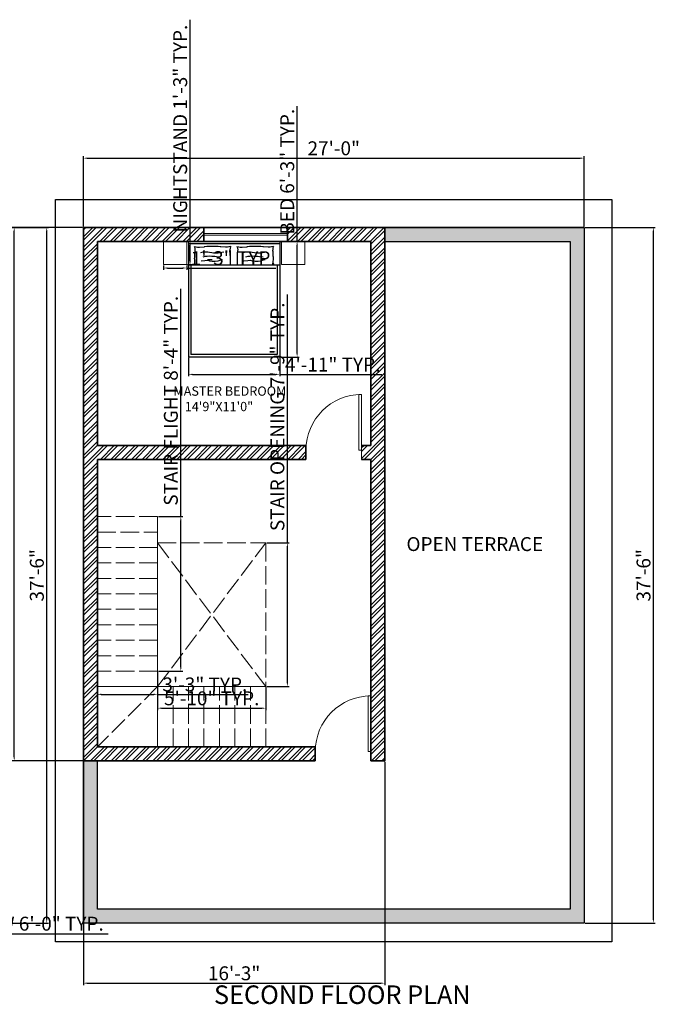
# Model space of a CAD drawing. Units: inches. Extents: x 638 to 1853, y 4393 to 5041.
# Tile 6 of 6: x 1441 to 1853, y 4404 to 5041. Entities that reach past the tile are written whole.
import ezdxf

# ---------------------------------------------------------------- set-up
doc = ezdxf.new("R2010")
doc.units = ezdxf.units.IN
doc.linetypes.add('ACAD_ISO02W100', pattern=[15, 12, -3])
for name, color, linetype, lineweight in [('A-ANNO-DIMS', 2, 'Continuous', 18), ('A-ANNO-TEXT', 7, 'Continuous', 25), ('A-AREA-IDEN', 7, 'Continuous', 18), ('A-DOOR', 4, 'Continuous', 18), ('A-FLOR-STRS', 7, 'Continuous', 18), ('A-FLOR-STRS-HIDN', 7, 'ACAD_ISO02W100', 18), ('A-FURN', 26, 'Continuous', 13), ('A-GLAZ', 5, 'Continuous', 18), ('A-WALL', 7, 'Continuous', 35), ('A-WALL-PATT', 251, 'Continuous', 13), ('A-WALL-PRPT', 7, 'Continuous', 25), ('A-WALL-PRPT-PATT', 141, 'Continuous', 13), ('C-PROP', 7, 'Continuous', 25)]:
    doc.layers.add(name, color=color, linetype=linetype, lineweight=lineweight)
doc.layers.add('supurgelik', color=31, linetype='Continuous')
doc.layers.add('TASLAR', color=32, linetype='Continuous')
doc.styles.get("Standard").update_dxf_attribs({"font": 'arial.ttf'})
doc.dimstyles.new('ISO-25', dxfattribs={"dimtxt": 9, "dimasz": 2.5, "dimexe": 1.25, "dimexo": 0.625, "dimtad": 1, "dimdec": 1, "dimlunit": 3, "dimtxsty": 'Standard', "dimcen": 2.5, "dimadec": 0, "dimazin": 0, "dimtfac": 1, "dimtdec": 1, "dimtmove": 0, "dimatfit": 3, "dimfxl": 1, "dimarcsym": 0})

# ---------------------------------------------------------------- blocks, each defined once
blk = doc.blocks.new('*U2')
for p, q in [((0, 0), (0, -6)), ((-36, 0), (-36, -6))]:
    blk.add_line(p, q)
blk.add_lwpolyline([(0, 0), (0, 36), (-1.75, 36), (-1.75, 0)], close=True)
blk.add_arc((0, 0), 36, 90, 180)
blk = doc.blocks.new('hgjgh')
at = {"layer": 'supurgelik'}
for p, q in [((85993.8, -4751.9), (85843.8, -4751.9)), ((85853.3, -4756.1), (85856.3, -4757)), ((85853.3, -4756.1), (85854.2, -4758.5)), ((85854.2, -4758.5), (85854.5, -4762.2)), ((85856.3, -4757), (85858.5, -4757.5)), ((85858.5, -4757.5), (85862.1, -4757.4)), ((85862.1, -4757.4), (85869.6, -4756.7)), ((85864.2, -4765.9), (85867.9, -4765)), ((85867.9, -4765), (85871.9, -4764.9)), ((85871.9, -4764.9), (85875.4, -4765.1)), ((85875.4, -4765.1), (85878.5, -4765.7)), ((85878.5, -4765.7), (85882, -4766.2)), ((85882, -4766.2), (85884.8, -4766.6)), ((85884.8, -4766.6), (85888.7, -4766.9)), ((85888.7, -4766.9), (85892.6, -4766.9)), ((85892.6, -4766.9), (85895.1, -4766.4)), ((85895.1, -4766.4), (85901.8, -4764.9)), ((85904.4, -4757.4), (85897, -4756.7)), ((85908, -4757.5), (85904.4, -4757.4)), ((85910.2, -4757), (85908, -4757.5)), ((85913.3, -4756.1), (85910.2, -4757)), ((85912.3, -4758.5), (85912, -4762.2)), ((85913.3, -4756.1), (85912.3, -4758.5)), ((85923.5, -4756.1), (85926.5, -4757)), ((85923.5, -4756.1), (85924.4, -4758.5)), ((85924.4, -4758.5), (85924.7, -4762.2)), ((85926.5, -4757), (85928.7, -4757.5)), ((85928.7, -4757.5), (85932.3, -4757.4)), ((85932.3, -4757.4), (85939.8, -4756.7)), ((85934.4, -4765.9), (85938.2, -4765)), ((85938.2, -4765), (85942.1, -4764.9)), ((85942.1, -4764.9), (85945.6, -4765.1)), ((85945.6, -4765.1), (85948.7, -4765.7)), ((85948.7, -4765.7), (85952.2, -4766.2)), ((85952.2, -4766.2), (85955, -4766.6)), ((85955, -4766.6), (85958.9, -4766.9)), ((85958.9, -4766.9), (85962.8, -4766.9)), ((85962.8, -4766.9), (85965.3, -4766.4)), ((85965.3, -4766.4), (85972, -4764.9)), ((85974.6, -4757.4), (85967.2, -4756.7)), ((85978.2, -4757.5), (85974.6, -4757.4)), ((85980.4, -4757), (85978.2, -4757.5)), ((85983.5, -4756.1), (85980.4, -4757)), ((85982.6, -4758.5), (85982.2, -4762.2)), ((85983.5, -4756.1), (85982.6, -4758.5)), ((85993.8, -4787.2), (85843.8, -4787.2)), ((85847.8, -4787.2), (85847.8, -4933.9)), ((85864.7, -4780.1), (85870.9, -4779.3)), ((85871.3, -4773), (85867.3, -4774)), ((85870.9, -4779.3), (85875.4, -4779)), ((85874.3, -4772.6), (85871.3, -4773)), ((85878.9, -4772.3), (85874.3, -4772.6)), ((85875.4, -4779), (85878.2, -4779.7)), ((85878.2, -4779.7), (85882.9, -4780.4)), ((85882, -4772.6), (85878.9, -4772.3)), ((85887, -4773), (85882, -4772.6)), ((85882.9, -4780.4), (85887.9, -4780.4)), ((85890.1, -4773.3), (85887, -4773)), ((85887.9, -4780.4), (85892.4, -4779.7)), ((85896.1, -4773.7), (85890.1, -4773.3)), ((85892.4, -4779.7), (85897, -4778.4)), ((85897, -4778.4), (85899.7, -4777.5)), ((85934.9, -4780.1), (85941.1, -4779.3)), ((85941.5, -4773), (85937.5, -4774)), ((85941.1, -4779.3), (85945.6, -4779)), ((85944.5, -4772.6), (85941.5, -4773)), ((85949.1, -4772.3), (85944.5, -4772.6)), ((85945.6, -4779), (85948.5, -4779.7)), ((85948.5, -4779.7), (85953.2, -4780.4)), ((85952.2, -4772.6), (85949.1, -4772.3)), ((85957.3, -4773), (85952.2, -4772.6)), ((85953.2, -4780.4), (85958.1, -4780.4)), ((85960.4, -4773.3), (85957.3, -4773)), ((85958.1, -4780.4), (85962.6, -4779.7)), ((85966.3, -4773.7), (85960.4, -4773.3)), ((85962.6, -4779.7), (85967.2, -4778.4)), ((85967.2, -4778.4), (85969.9, -4777.5)), ((85989.8, -4787.2), (85989.8, -4933.9)), ((85989.8, -4933.9), (85847.8, -4933.9))]:
    blk.add_line(p, q, dxfattribs=at)
for centre, radius, start, end in [((85954.1, -4776.1), 100.7, 175.3005, 180), ((85905.8, -4772.1), 52.3, 169.0896, 175.3005), ((85877.4, -4828.5), 72.2, 95.1362, 96.1932), ((85883.3, -4894.2), 138.1, 90, 95.1362), ((85883.3, -4894.2), 138.1, 84.8638, 90), ((85889.2, -4828.5), 72.2, 83.8068, 84.8638), ((85860.7, -4772.1), 52.3, 4.6995, 10.9104), ((85812.4, -4776.1), 100.7, 0, 4.6995), ((86024.3, -4776.1), 100.7, 175.3005, 180), ((85976, -4772.1), 52.3, 169.0896, 175.3005), ((85947.6, -4828.5), 72.2, 95.1362, 96.1932), ((85953.5, -4894.2), 138.1, 90, 95.1362), ((85953.5, -4894.2), 138.1, 84.8638, 90), ((85959.4, -4828.5), 72.2, 83.8068, 84.8638), ((85930.9, -4772.1), 52.3, 4.6995, 10.9104), ((85882.6, -4776.1), 100.7, 0, 4.6995), ((85954.1, -4776.1), 100.7, 180, 184.6995), ((85905.8, -4780), 52.3, 184.6995, 187.8973), ((85860.7, -4780), 52.3, 352.1027, 355.3005), ((85812.4, -4776.1), 100.7, 355.3005, 0), ((86024.3, -4776.1), 100.7, 180, 184.6995), ((85976, -4780), 52.3, 184.6995, 187.8973), ((85930.9, -4780), 52.3, 352.1027, 355.3005), ((85882.6, -4776.1), 100.7, 355.3005, 0)]:
    blk.add_arc(centre, radius, start, end, dxfattribs=at)
at = {"layer": 'TASLAR'}
for p, q in [((85843.8, -4747.9), (85843.8, -4937.9)), ((85993.8, -4747.9), (85843.8, -4747.9)), ((85993.8, -4747.9), (85993.8, -4937.9)), ((85993.8, -4937.9), (85843.8, -4937.9))]:
    blk.add_line(p, q, dxfattribs=at)
blk = doc.blocks.new('BED-NIGHTSTAND-15')
blk.add_lwpolyline([(0, 14.98), (14.98, 14.98), (14.98, 0), (0, 0)], close=True)
blk = doc.blocks.new('WINDOW-GLAZING-54IN')
for p, q in [((0, 1), (54, 1)), ((0, 0), (54, 0))]:
    blk.add_line(p, q)
blk = doc.blocks.new('STAIR-WELL-OPENING')
for p, q in [((0, 93), (70, 0)), ((0, 0), (70, 93))]:
    blk.add_line(p, q)
blk.add_lwpolyline([(0, 93), (70, 93), (70, 0), (0, 0)], close=True)
blk = doc.blocks.new('STAIR-RUN-BEYOND')
for p, q in [((39, 100), (0, 100)), ((0, 90), (39, 90)), ((39, 80), (0, 80)), ((39, 70), (0, 70)), ((39, 60), (0, 60)), ((39, 50), (0, 50)), ((39, 40), (0, 40)), ((39, 30), (0, 30)), ((39, 20), (0, 20)), ((39, 10), (0, 10)), ((39, 0), (0, 0)), ((39, 0), (0, 0))]:
    blk.add_line(p, q)
blk = doc.blocks.new('*D34')
at = {"layer": 'A-ANNO-DIMS', "color": 0, "lineweight": -2, "transparency": 16777216}
for p, q in [((1620.93, 4897.19), (1620.93, 4984.75)), ((1610.33, 4897.19), (1622.18, 4897.19)), ((1620.93, 4824.89), (1620.93, 4894.69)), ((1610.33, 4822.39), (1622.18, 4822.39))]:
    blk.add_line(p, q, dxfattribs=at)
at = {"layer": 'A-ANNO-DIMS', "color": 0, "transparency": 16777216}
for points in [[(1620.51, 4894.69), (1621.35, 4894.69), (1620.93, 4897.19)], [(1620.51, 4824.89), (1621.35, 4824.89), (1620.93, 4822.39)]]:
    blk.add_solid(points, dxfattribs=at)
at = {"layer": 'Defpoints', "color": 0, "transparency": 16777216}
for p in [(1609.71, 4897.19), (1620.93, 4897.19), (1609.71, 4822.39)]:
    blk.add_point(p, dxfattribs=at)
at = {"layer": 'A-ANNO-DIMS', "color": 0, "transparency": 16777216, "insert": (1615.71, 4942.22), "char_height": 9, "attachment_point": 5, "rotation": 90}
blk.add_mtext('BED 6\'-3" TYP.', dxfattribs=at)
blk = doc.blocks.new('*D35')
at = {"layer": 'A-ANNO-DIMS', "color": 0, "lineweight": -2, "transparency": 16777216}
for p, q in [((1550.65, 4821.77), (1550.65, 4809.92)), ((1609.71, 4821.77), (1609.71, 4809.92)), ((1553.15, 4811.17), (1607.21, 4811.17)), ((1609.71, 4811.17), (1675.67, 4811.17))]:
    blk.add_line(p, q, dxfattribs=at)
at = {"layer": 'A-ANNO-DIMS', "color": 0, "transparency": 16777216}
for points in [[(1553.15, 4811.59), (1553.15, 4810.75), (1550.65, 4811.17)], [(1607.21, 4811.59), (1607.21, 4810.75), (1609.71, 4811.17)]]:
    blk.add_solid(points, dxfattribs=at)
at = {"layer": 'Defpoints', "color": 0, "transparency": 16777216}
for p in [(1550.65, 4822.39), (1609.71, 4822.39), (1609.71, 4811.17)]:
    blk.add_point(p, dxfattribs=at)
at = {"layer": 'A-ANNO-DIMS', "color": 0, "transparency": 16777216, "insert": (1643.94, 4816.32), "char_height": 9, "attachment_point": 5}
blk.add_mtext('4\'-11" TYP.', dxfattribs=at)
blk = doc.blocks.new('*D36')
at = {"layer": 'A-ANNO-DIMS', "color": 0, "lineweight": -2, "transparency": 16777216}
for p, q in [((1551.72, 4897.19), (1551.72, 5040.59)), ((1550.1, 4897.19), (1552.97, 4897.19)), ((1551.72, 4884.71), (1551.72, 4894.69)), ((1550.1, 4882.21), (1552.97, 4882.21))]:
    blk.add_line(p, q, dxfattribs=at)
at = {"layer": 'A-ANNO-DIMS', "color": 0, "transparency": 16777216}
for points in [[(1551.3, 4894.69), (1552.14, 4894.69), (1551.72, 4897.19)], [(1551.3, 4884.71), (1552.14, 4884.71), (1551.72, 4882.21)]]:
    blk.add_solid(points, dxfattribs=at)
at = {"layer": 'Defpoints', "color": 0, "transparency": 16777216}
for p in [(1549.47, 4897.19), (1551.72, 4897.19), (1549.47, 4882.21)]:
    blk.add_point(p, dxfattribs=at)
at = {"layer": 'A-ANNO-DIMS', "color": 0, "transparency": 16777216, "insert": (1546.44, 4970.14), "char_height": 9, "attachment_point": 5, "rotation": 90}
blk.add_mtext('NIGHTSTAND 1\'-3" TYP.', dxfattribs=at)
blk = doc.blocks.new('*D37')
at = {"layer": 'A-ANNO-DIMS', "color": 0, "lineweight": -2, "transparency": 16777216}
for p, q in [((1534.49, 4881.58), (1534.49, 4878.71)), ((1536.99, 4879.96), (1546.97, 4879.96)), ((1549.47, 4881.58), (1549.47, 4878.71)), ((1549.47, 4879.96), (1607.24, 4879.96))]:
    blk.add_line(p, q, dxfattribs=at)
at = {"layer": 'A-ANNO-DIMS', "color": 0, "transparency": 16777216}
for points in [[(1536.99, 4880.38), (1536.99, 4879.55), (1534.49, 4879.96)], [(1546.97, 4880.38), (1546.97, 4879.55), (1549.47, 4879.96)]]:
    blk.add_solid(points, dxfattribs=at)
at = {"layer": 'Defpoints', "color": 0, "transparency": 16777216}
for p in [(1534.49, 4882.21), (1549.47, 4882.21), (1549.47, 4879.96)]:
    blk.add_point(p, dxfattribs=at)
at = {"layer": 'A-ANNO-DIMS', "color": 0, "transparency": 16777216, "insert": (1579.6, 4885.19), "char_height": 9, "attachment_point": 5}
blk.add_mtext('1\'-3" TYP.', dxfattribs=at)
blk = doc.blocks.new('*D52')
at = {"layer": 'A-ANNO-DIMS', "color": 0, "lineweight": -2, "transparency": 16777216}
for p, q in [((1614.63, 4702.19), (1614.63, 4862.76)), ((1601.31, 4702.19), (1615.88, 4702.19)), ((1614.63, 4611.69), (1614.63, 4699.69)), ((1601.31, 4609.19), (1615.88, 4609.19))]:
    blk.add_line(p, q, dxfattribs=at)
at = {"layer": 'A-ANNO-DIMS', "color": 0, "transparency": 16777216}
for points in [[(1614.22, 4699.69), (1615.05, 4699.69), (1614.63, 4702.19)], [(1614.22, 4611.69), (1615.05, 4611.69), (1614.63, 4609.19)]]:
    blk.add_solid(points, dxfattribs=at)
at = {"layer": 'Defpoints', "color": 0, "transparency": 16777216}
for p in [(1600.68, 4702.19), (1614.63, 4702.19), (1600.68, 4609.19)]:
    blk.add_point(p, dxfattribs=at)
at = {"layer": 'A-ANNO-DIMS', "color": 0, "transparency": 16777216, "insert": (1609.35, 4783.73), "char_height": 9, "attachment_point": 5, "rotation": 90}
blk.add_mtext('STAIR OPENING 7\'-9" TYP.', dxfattribs=at)
blk = doc.blocks.new('*D53')
at = {"layer": 'A-ANNO-DIMS', "color": 0, "lineweight": -2, "transparency": 16777216}
for p, q in [((1530.68, 4608.57), (1530.68, 4593.99)), ((1600.68, 4608.57), (1600.68, 4593.99)), ((1533.18, 4595.24), (1598.18, 4595.24))]:
    blk.add_line(p, q, dxfattribs=at)
at = {"layer": 'A-ANNO-DIMS', "color": 0, "transparency": 16777216}
for points in [[(1533.18, 4595.66), (1533.18, 4594.83), (1530.68, 4595.24)], [(1598.18, 4595.66), (1598.18, 4594.83), (1600.68, 4595.24)]]:
    blk.add_solid(points, dxfattribs=at)
at = {"layer": 'Defpoints', "color": 0, "transparency": 16777216}
for p in [(1530.68, 4609.19), (1600.68, 4609.19), (1600.68, 4595.24)]:
    blk.add_point(p, dxfattribs=at)
at = {"layer": 'A-ANNO-DIMS', "color": 0, "transparency": 16777216, "insert": (1565.68, 4600.46), "char_height": 9, "attachment_point": 5}
blk.add_mtext('5\'-10" TYP.', dxfattribs=at)
blk = doc.blocks.new('*D54')
at = {"layer": 'A-ANNO-DIMS', "color": 0, "lineweight": -2, "transparency": 16777216}
for p, q in [((1309.08, 4459.57), (1309.08, 4448.14)), ((1381.08, 4459.57), (1381.08, 4448.14)), ((1311.58, 4449.39), (1378.58, 4449.39)), ((1381.08, 4449.39), (1498.72, 4449.39))]:
    blk.add_line(p, q, dxfattribs=at)
at = {"layer": 'A-ANNO-DIMS', "color": 0, "transparency": 16777216}
for points in [[(1311.58, 4449.81), (1311.58, 4448.98), (1309.08, 4449.39)], [(1378.58, 4449.81), (1378.58, 4448.98), (1381.08, 4449.39)]]:
    blk.add_solid(points, dxfattribs=at)
at = {"layer": 'Defpoints', "color": 0, "transparency": 16777216}
for p in [(1309.08, 4460.19), (1381.08, 4460.19), (1381.08, 4449.39)]:
    blk.add_point(p, dxfattribs=at)
at = {"layer": 'A-ANNO-DIMS', "color": 0, "transparency": 16777216, "insert": (1441.15, 4454.68), "char_height": 9, "attachment_point": 5}
blk.add_mtext('WINDOW 6\'-0" TYP.', dxfattribs=at)
blk = doc.blocks.new('*D60')
at = {"layer": 'A-ANNO-DIMS', "color": 0, "lineweight": -2, "transparency": 16777216}
for p, q in [((1545.68, 4719.19), (1545.68, 4866.48)), ((1531.31, 4719.19), (1546.93, 4719.19)), ((1545.68, 4621.69), (1545.68, 4716.69)), ((1531.31, 4619.19), (1546.93, 4619.19))]:
    blk.add_line(p, q, dxfattribs=at)
at = {"layer": 'A-ANNO-DIMS', "color": 0, "transparency": 16777216}
for points in [[(1545.27, 4716.69), (1546.1, 4716.69), (1545.68, 4719.19)], [(1545.27, 4621.69), (1546.1, 4621.69), (1545.68, 4619.19)]]:
    blk.add_solid(points, dxfattribs=at)
at = {"layer": 'Defpoints', "color": 0, "transparency": 16777216}
for p in [(1530.68, 4719.19), (1545.68, 4719.19), (1530.68, 4619.19)]:
    blk.add_point(p, dxfattribs=at)
at = {"layer": 'A-ANNO-DIMS', "color": 0, "transparency": 16777216, "insert": (1540.4, 4794.09), "char_height": 9, "attachment_point": 5, "rotation": 90}
blk.add_mtext('STAIR FLIGHT 8\'-4" TYP.', dxfattribs=at)
blk = doc.blocks.new('*D61')
at = {"layer": 'A-ANNO-DIMS', "color": 0, "lineweight": -2, "transparency": 16777216}
for p, q in [((1491.68, 4618.57), (1491.68, 4602.94)), ((1530.68, 4618.57), (1530.68, 4602.94)), ((1494.18, 4604.19), (1528.18, 4604.19)), ((1530.68, 4604.19), (1589.29, 4604.19))]:
    blk.add_line(p, q, dxfattribs=at)
at = {"layer": 'A-ANNO-DIMS', "color": 0, "transparency": 16777216}
for points in [[(1494.18, 4604.61), (1494.18, 4603.78), (1491.68, 4604.19)], [(1528.18, 4604.61), (1528.18, 4603.78), (1530.68, 4604.19)]]:
    blk.add_solid(points, dxfattribs=at)
at = {"layer": 'Defpoints', "color": 0, "transparency": 16777216}
for p in [(1491.68, 4619.19), (1530.68, 4619.19), (1530.68, 4604.19)]:
    blk.add_point(p, dxfattribs=at)
at = {"layer": 'A-ANNO-DIMS', "color": 0, "transparency": 16777216, "insert": (1561.23, 4609.42), "char_height": 9, "attachment_point": 5}
blk.add_mtext('3\'-3" TYP.', dxfattribs=at)
blk = doc.blocks.new('*D89')
at = {"layer": 'A-ANNO-DIMS', "color": 0, "lineweight": -2, "transparency": 16777216}
for p, q in [((1414.71, 4906.19), (1460.16, 4906.19)), ((1458.91, 4458.69), (1458.91, 4903.69)), ((1414.71, 4456.19), (1460.16, 4456.19))]:
    blk.add_line(p, q, dxfattribs=at)
at = {"layer": 'A-ANNO-DIMS', "color": 0, "transparency": 16777216}
for points in [[(1458.49, 4903.69), (1459.32, 4903.69), (1458.91, 4906.19)], [(1458.49, 4458.69), (1459.32, 4458.69), (1458.91, 4456.19)]]:
    blk.add_solid(points, dxfattribs=at)
at = {"layer": 'Defpoints', "color": 0, "transparency": 16777216}
for p in [(1414.08, 4906.19), (1458.91, 4906.19), (1414.08, 4456.19)]:
    blk.add_point(p, dxfattribs=at)
at = {"layer": 'A-ANNO-DIMS', "color": 0, "transparency": 16777216, "insert": (1453.68, 4681.19), "char_height": 9, "attachment_point": 5, "rotation": 90}
blk.add_mtext('37\'-6"', dxfattribs=at)
blk = doc.blocks.new('*D94')
at = {"layer": 'A-ANNO-DIMS', "color": 0, "lineweight": -2, "transparency": 16777216}
for p, q in [((1482.68, 4906.82), (1482.68, 4952.27)), ((1485.18, 4951.02), (1804.18, 4951.02)), ((1806.68, 4906.82), (1806.68, 4952.27))]:
    blk.add_line(p, q, dxfattribs=at)
at = {"layer": 'A-ANNO-DIMS', "color": 0, "transparency": 16777216}
for points in [[(1485.18, 4951.44), (1485.18, 4950.6), (1482.68, 4951.02)], [(1804.18, 4951.44), (1804.18, 4950.6), (1806.68, 4951.02)]]:
    blk.add_solid(points, dxfattribs=at)
at = {"layer": 'Defpoints', "color": 0, "transparency": 16777216}
for p in [(1806.68, 4951.02), (1482.68, 4906.19), (1806.68, 4906.19)]:
    blk.add_point(p, dxfattribs=at)
at = {"layer": 'A-ANNO-DIMS', "color": 0, "transparency": 16777216, "insert": (1644.68, 4956.24), "char_height": 9, "attachment_point": 5}
blk.add_mtext('27\'-0"', dxfattribs=at)
blk = doc.blocks.new('*D95')
at = {"layer": 'A-ANNO-DIMS', "color": 0, "lineweight": -2, "transparency": 16777216}
for p, q in [((1807.31, 4906.19), (1852.76, 4906.19)), ((1851.51, 4458.69), (1851.51, 4903.69)), ((1807.31, 4456.19), (1852.76, 4456.19))]:
    blk.add_line(p, q, dxfattribs=at)
at = {"layer": 'A-ANNO-DIMS', "color": 0, "transparency": 16777216}
for points in [[(1851.09, 4903.69), (1851.92, 4903.69), (1851.51, 4906.19)], [(1851.09, 4458.69), (1851.92, 4458.69), (1851.51, 4456.19)]]:
    blk.add_solid(points, dxfattribs=at)
at = {"layer": 'Defpoints', "color": 0, "transparency": 16777216}
for p in [(1806.68, 4906.19), (1851.51, 4906.19), (1806.68, 4456.19)]:
    blk.add_point(p, dxfattribs=at)
at = {"layer": 'A-ANNO-DIMS', "color": 0, "transparency": 16777216, "insert": (1846.28, 4681.19), "char_height": 9, "attachment_point": 5, "rotation": 90}
blk.add_mtext('37\'-6"', dxfattribs=at)
blk = doc.blocks.new('*D96')
at = {"layer": 'A-ANNO-DIMS', "color": 0, "lineweight": -2, "transparency": 16777216}
for p, q in [((1482.68, 4560.57), (1482.68, 4416.12)), ((1677.68, 4560.57), (1677.68, 4416.12)), ((1485.18, 4417.37), (1675.18, 4417.37))]:
    blk.add_line(p, q, dxfattribs=at)
at = {"layer": 'A-ANNO-DIMS', "color": 0, "transparency": 16777216}
for points in [[(1485.18, 4417.79), (1485.18, 4416.95), (1482.68, 4417.37)], [(1675.18, 4417.79), (1675.18, 4416.95), (1677.68, 4417.37)]]:
    blk.add_solid(points, dxfattribs=at)
at = {"layer": 'Defpoints', "color": 0, "transparency": 16777216}
for p in [(1482.68, 4561.19), (1677.68, 4561.19), (1677.68, 4417.37)]:
    blk.add_point(p, dxfattribs=at)
at = {"layer": 'A-ANNO-DIMS', "color": 0, "transparency": 16777216, "insert": (1580.18, 4422.59), "char_height": 9, "attachment_point": 5}
blk.add_mtext('16\'-3"', dxfattribs=at)
blk = doc.blocks.new('*D97')
at = {"layer": 'A-ANNO-DIMS', "color": 0, "lineweight": -2, "transparency": 16777216}
for p, q in [((1482.06, 4906.19), (1436.61, 4906.19)), ((1437.86, 4563.69), (1437.86, 4903.69)), ((1482.06, 4561.19), (1436.61, 4561.19))]:
    blk.add_line(p, q, dxfattribs=at)
at = {"layer": 'A-ANNO-DIMS', "color": 0, "transparency": 16777216}
for points in [[(1437.44, 4903.69), (1438.27, 4903.69), (1437.86, 4906.19)], [(1437.44, 4563.69), (1438.27, 4563.69), (1437.86, 4561.19)]]:
    blk.add_solid(points, dxfattribs=at)
at = {"layer": 'Defpoints', "color": 0, "transparency": 16777216}
for p in [(1437.86, 4906.19), (1482.68, 4906.19), (1482.68, 4561.19)]:
    blk.add_point(p, dxfattribs=at)
at = {"layer": 'A-ANNO-DIMS', "color": 0, "transparency": 16777216, "insert": (1432.64, 4733.69), "char_height": 9, "attachment_point": 5, "rotation": 90}
blk.add_mtext('28\'-9"', dxfattribs=at)

msp = doc.modelspace()

# ---------------------------------------------------------------- hatches: boundary and pattern name
at = {"layer": 'A-WALL-PATT', "transparency": 33554687}
h = msp.add_hatch(dxfattribs=at)
h.set_pattern_fill('ANSI32', color=256, scale=0.5)
h.set_pattern_definition([(45, (-130.6875, 0), (-3.367596, 3.367596), []), (45, (-128.4424, 0), (-3.367596, 3.367596), [])])
h.paths.add_polyline_path([(1482.68, 4561.19), (1632.68, 4561.19), (1632.68, 4567.19), (1632.68, 4570.19), (1491.68, 4570.19), (1491.68, 4756.19), (1626.68, 4756.19), (1626.68, 4762.19), (1626.68, 4765.19), (1491.68, 4765.19), (1491.68, 4897.19), (1560.68, 4897.19), (1560.68, 4906.19), (1482.68, 4906.19)])
h.paths.add_polyline_path([(1668.68, 4765.19), (1662.68, 4765.19), (1662.68, 4762.19), (1662.68, 4756.19), (1668.68, 4756.19), (1668.68, 4561.19), (1677.68, 4561.19), (1677.68, 4906.19), (1614.68, 4906.19), (1614.68, 4897.19), (1668.68, 4897.19)])
at = {"layer": 'A-WALL-PRPT-PATT', "transparency": 33554687}
h = msp.add_hatch(color=256, dxfattribs=at)
h.dxf.hatch_style = 1
h.paths.add_polyline_path([(1491.68, 4561.19), (1482.68, 4561.19), (1482.68, 4456.19), (1806.68, 4456.19), (1806.68, 4906.19), (1677.68, 4906.19), (1677.68, 4897.19), (1797.68, 4897.19), (1797.68, 4465.19), (1491.68, 4465.19)])

# ---------------------------------------------------------------- linework, layer by layer
at = {"layer": 'A-FLOR-STRS'}
for p, q in [((1530.68, 4570.19), (1530.68, 4719.19)), ((1600.68, 4609.19), (1491.68, 4609.19))]:
    msp.add_line(p, q, dxfattribs=at)
at = {"layer": 'A-FLOR-STRS-HIDN'}
for p, q in [((1530.68, 4609.19), (1491.68, 4570.19)), ((1540.68, 4570.19), (1540.68, 4609.19)), ((1550.68, 4570.19), (1550.68, 4609.19)), ((1560.68, 4570.19), (1560.68, 4609.19)), ((1570.68, 4570.19), (1570.68, 4609.19)), ((1580.68, 4570.19), (1580.68, 4609.19)), ((1590.68, 4570.19), (1590.68, 4609.19)), ((1600.68, 4570.19), (1600.68, 4609.19))]:
    msp.add_line(p, q, dxfattribs=at)
at = {"layer": 'A-WALL'}
for p, q in [((1482.68, 4906.19), (1806.68, 4906.19)), ((1482.68, 4456.19), (1482.68, 4906.19)), ((1560.68, 4897.19), (1560.68, 4906.19)), ((1614.68, 4897.19), (1614.68, 4906.19)), ((1677.68, 4561.19), (1677.68, 4906.19)), ((1491.68, 4897.19), (1668.68, 4897.19)), ((1491.68, 4765.19), (1491.68, 4897.19)), ((1668.68, 4765.19), (1668.68, 4897.19)), ((1491.68, 4765.19), (1626.68, 4765.19)), ((1626.68, 4756.19), (1626.68, 4765.19)), ((1662.68, 4765.19), (1668.68, 4765.19)), ((1491.68, 4570.19), (1491.68, 4756.19)), ((1491.68, 4756.19), (1626.68, 4756.19)), ((1662.68, 4756.19), (1668.68, 4756.19)), ((1668.68, 4561.19), (1668.68, 4756.19)), ((1632.68, 4570.19), (1491.68, 4570.19)), ((1632.68, 4561.19), (1632.68, 4570.19)), ((1632.68, 4561.19), (1482.68, 4561.19)), ((1677.68, 4561.19), (1668.68, 4561.19))]:
    msp.add_line(p, q, dxfattribs=at)
at = {"layer": 'A-WALL-PRPT'}
for p, q in [((1806.68, 4906.19), (1806.68, 4456.19)), ((1677.68, 4897.19), (1797.68, 4897.19)), ((1797.68, 4897.19), (1797.68, 4465.19)), ((1491.68, 4465.19), (1491.68, 4561.19)), ((1797.68, 4465.19), (1491.68, 4465.19)), ((1806.68, 4456.19), (1482.68, 4456.19))]:
    msp.add_line(p, q, dxfattribs=at)
at = {"layer": 'C-PROP'}
msp.add_lwpolyline([(1464.68, 4924.19), (1824.68, 4924.19), (1824.68, 4444.19), (1464.68, 4444.19)], close=True, dxfattribs=at)

# ---------------------------------------------------------------- block references
at = {"layer": 'A-DOOR'}
for p in [(1662.68, 4762.19), (1668.68, 4567.19)]:
    msp.add_blockref('*U2', p, dxfattribs=at)
at = {"layer": 'A-FLOR-STRS-HIDN'}
for name, p in [('STAIR-RUN-BEYOND', (1491.68, 4619.19)), ('STAIR-WELL-OPENING', (1530.68, 4609.19))]:
    msp.add_blockref(name, p, dxfattribs=at)
at = {"layer": 'A-FURN'}
for p in [(1534.49, 4882.21), (1610.89, 4882.21)]:
    msp.add_blockref('BED-NIGHTSTAND-15', p, dxfattribs=at)
at = {"layer": 'A-FURN', "xscale": 0.393701, "yscale": 0.393701, "zscale": 0.393701}
msp.add_blockref('hgjgh', (-32246.14, 6766.44), dxfattribs=at)
at = {"layer": 'A-GLAZ', "rotation": 180}
msp.add_blockref('WINDOW-GLAZING-54IN', (1614.68, 4902.19), dxfattribs=at)

# ---------------------------------------------------------------- texts
at = {"layer": 'A-ANNO-TEXT', "insert": (1567.14, 4415.91), "char_height": 12, "attachment_point": 1}
msp.add_mtext_dynamic_manual_height_columns('SECOND FLOOR PLAN', width=193.1285, gutter_width=12.5, heights=[0], dxfattribs=at)
at = {"layer": 'A-AREA-IDEN', "attachment_point": 1}
for s, insert, char_height in [('MASTER BEDROOM\\P    14\'9"X11\'0"', (1540.91, 4803.35), 6), ('OPEN TERRACE', (1691.69, 4705.88), 9)]:
    msp.add_mtext_dynamic_manual_height_columns(s, width=125.7999, gutter_width=12.5, heights=[0], dxfattribs=dict(at, insert=insert, char_height=char_height))

# ---------------------------------------------------------------- dimensions: what is measured, and where the dimension line sits
at = {"layer": 'A-ANNO-DIMS'}
for base, p1, p2, angle, text, picture, middle in [((1551.72, 4897.19), (1549.47, 4882.21), (1549.47, 4897.19), 90, 'NIGHTSTAND <> TYP.', '*D36', (1546.44, 4970.14)), ((1620.93, 4897.19), (1609.71, 4822.39), (1609.71, 4897.19), 90, 'BED <> TYP.', '*D34', (1615.71, 4942.22)), ((1545.68, 4719.19), (1530.68, 4619.19), (1530.68, 4719.19), 90, 'STAIR FLIGHT <> TYP.', '*D60', (1540.4, 4794.09)), ((1614.63, 4702.19), (1600.68, 4609.19), (1600.68, 4702.19), 90, 'STAIR OPENING <> TYP.', '*D52', (1609.35, 4783.73)), ((1381.08, 4449.39), (1309.08, 4460.19), (1381.08, 4460.19), 0, 'WINDOW <> TYP.', '*D54', (1441.15, 4454.68))]:
    dim = msp.add_linear_dim(base=base, p1=p1, p2=p2, angle=angle, text=text, dimstyle='ISO-25', override={"dimdec": 1, "dimlfac": 1, "dimrnd": 0, "dimzin": 1, "dimdsep": 46, "dimlunit": 4, "dimfrac": 2}, dxfattribs=at)
    dim.commit()
    dim.dimension.update_dxf_attribs({"geometry": picture, "text_midpoint": middle})
for base, p1, p2, picture, middle in [((1806.68, 4951.02), (1482.68, 4906.19), (1806.68, 4906.19), '*D94', (1644.68, 4956.24)), ((1677.68, 4417.37), (1482.68, 4561.19), (1677.68, 4561.19), '*D96', (1580.18, 4422.59))]:
    dim = msp.add_linear_dim(base=base, p1=p1, p2=p2, dimstyle='ISO-25', override={"dimdec": 1, "dimlfac": 1, "dimrnd": 0, "dimzin": 1, "dimdsep": 46, "dimlunit": 4, "dimfrac": 2}, dxfattribs=at)
    dim.commit()
    dim.dimension.update_dxf_attribs({"geometry": picture, "text_midpoint": middle})
for base, p1, p2, picture, middle in [((1458.91, 4906.19), (1414.08, 4456.19), (1414.08, 4906.19), '*D89', (1453.68, 4681.19)), ((1437.86, 4906.19), (1482.68, 4561.19), (1482.68, 4906.19), '*D97', (1432.64, 4733.69)), ((1851.51, 4906.19), (1806.68, 4456.19), (1806.68, 4906.19), '*D95', (1846.28, 4681.19))]:
    dim = msp.add_linear_dim(base=base, p1=p1, p2=p2, angle=90, dimstyle='ISO-25', override={"dimdec": 1, "dimlfac": 1, "dimrnd": 0, "dimzin": 1, "dimdsep": 46, "dimlunit": 4, "dimfrac": 2}, dxfattribs=at)
    dim.commit()
    dim.dimension.update_dxf_attribs({"geometry": picture, "text_midpoint": middle})
for base, p1, p2, picture, middle in [((1549.47, 4879.96), (1534.49, 4882.21), (1549.47, 4882.21), '*D37', (1579.6, 4885.19)), ((1609.71, 4811.17), (1550.65, 4822.39), (1609.71, 4822.39), '*D35', (1643.94, 4816.32)), ((1530.68, 4604.19), (1491.68, 4619.19), (1530.68, 4619.19), '*D61', (1561.23, 4609.42)), ((1600.68, 4595.24), (1530.68, 4609.19), (1600.68, 4609.19), '*D53', (1565.68, 4600.46))]:
    dim = msp.add_linear_dim(base=base, p1=p1, p2=p2, text='<> TYP.', dimstyle='ISO-25', override={"dimdec": 1, "dimlfac": 1, "dimrnd": 0, "dimzin": 1, "dimdsep": 46, "dimlunit": 4, "dimfrac": 2}, dxfattribs=at)
    dim.commit()
    dim.dimension.update_dxf_attribs({"geometry": picture, "text_midpoint": middle})

doc.saveas('drawing.dxf')
